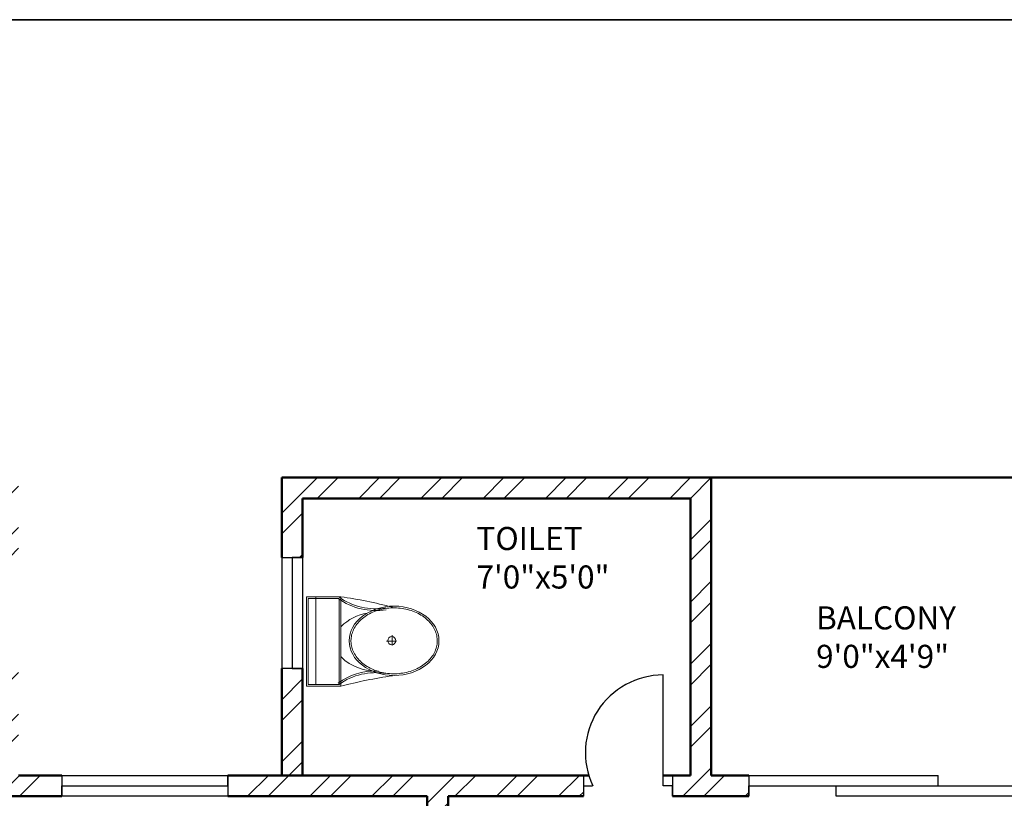
# Model space of a CAD drawing. Units: inches. Extents: x 963 to 2075, y 289 to 2657.
# Tile 97 of 98: x 1672 to 1885, y 2489 to 2657. Entities that reach past the tile are written whole.
import ezdxf

# ---------------------------------------------------------------- set-up
doc = ezdxf.new("R2010")
doc.units = ezdxf.units.IN
for name, color, linetype, lineweight in [('A-ANNO-TTLB', 7, 'Continuous', 35), ('A-AREA-IDEN', 7, 'Continuous', 18), ('A-DOOR', 4, 'Continuous', 25), ('A-FLOR-FIXT', 9, 'Continuous', 18), ('A-GLAZ', 3, 'Continuous', 25), ('A-WALL', 7, 'Continuous', 50), ('A-WALL-PATT', 8, 'Continuous', 13)]:
    doc.layers.add(name, color=color, linetype=linetype, lineweight=lineweight)
doc.styles.get("Standard").update_dxf_attribs({"font": 'arial.ttf'})

# ---------------------------------------------------------------- blocks, each defined once
blk = doc.blocks.new('A$C31115884')
for p, q in [((257.5, 466.4), (257.5, 523.2)), ((283.1, 497.7), (223.4, 497.7)), ((0, 200), (0, 0)), ((520, 200), (0, 200)), ((10, 190), (10, 10)), ((510, 190), (10, 190)), ((510, 10), (510, 190)), ((520, 0), (520, 200)), ((510, 54.5), (0, 54.5)), ((10, 10), (510, 10)), ((0, 0), (520, 0))]:
    blk.add_line(p, q)
blk.add_circle((255.6, 496.4), 23.6)
for centre, radius, start, end in [((2777.7, -204.6), 2807, 165.4549, 171.7133), ((-294.5, 403.3), 364.7, 324.2091, 9.3499), ((-294.5, 403.3), 374.7, 324.2091, 9.3499), ((805.8, 403.3), 364.7, 170.6501, 215.7909), ((3237, 905), 2807, 188.2867, 194.5451), ((139.5, 406.2), 293.5, 315.8436, 2.6563), ((805.8, 403.3), 374.7, 179.2036, 215.7909), ((383.6, 406.2), 293.5, 190.2774, 224.1564)]:
    blk.add_arc(centre, radius, start, end)
blk.add_ellipse((256.2, 509.9), major_axis=(0, -260.7), ratio=0.772727)
blk.add_open_spline([(256.2, 259.2), (263.1, 259.2), (270, 259.7), (287.8, 262.3), (298.7, 265.1), (319.9, 273.1), (330.2, 278.4), (350.1, 291.1), (359.7, 298.7), (377.7, 315.9), (386.2, 325.5), (401.7, 346.6), (408.8, 358.1), (421.3, 382.5), (426.8, 395.5), (435.9, 422.4), (439.5, 436.4), (444.8, 465.1), (446.5, 479.7), (447.9, 509.2), (447.6, 524), (445, 553.3), (442.7, 567.8), (436.3, 596), (432.1, 609.7), (421.9, 636), (416, 648.6), (402.5, 672.1), (395, 683), (378.6, 703), (369.8, 712.1), (351.1, 728), (341.3, 734.8), (320.9, 746.2), (310.4, 750.7), (288.9, 757.3), (278, 759.4), (256, 761), (245, 760.6), (223.1, 757.2), (212.3, 754.3), (191.1, 746.1), (180.8, 740.7), (160.9, 727.8), (151.4, 720.1), (133.5, 702.7), (125.1, 693), (109.6, 671.7), (102.6, 660.2), (90.2, 635.7), (84.9, 622.7), (76, 595.6), (72.4, 581.6), (67.2, 552.9), (65.6, 538.2), (64.4, 508.8), (64.8, 494), (67.5, 464.7), (69.9, 450.2), (76.6, 422), (80.8, 408.3), (91.1, 382.2), (97.2, 369.7), (110.8, 346.3), (118.4, 335.4), (134.8, 315.6), (143.7, 306.7), (162.4, 290.9), (172.3, 284.2), (192.8, 273), (203.3, 268.6), (224.8, 262.2), (235.8, 260.2), (249.9, 259.3), (253, 259.2), (256.2, 259.2)], degree=3, knots=[0, 0, 0, 0, 0.110105, 0.110105, 0.285049, 0.285049, 0.459994, 0.459994, 0.634938, 0.634938, 0.809882, 0.809882, 0.984827, 0.984827, 1.159771, 1.159771, 1.334715, 1.334715, 1.50966, 1.50966, 1.684604, 1.684604, 1.859549, 1.859549, 2.034493, 2.034493, 2.209437, 2.209437, 2.384382, 2.384382, 2.559326, 2.559326, 2.73427, 2.73427, 2.909215, 2.909215, 3.084159, 3.084159, 3.259103, 3.259103, 3.434048, 3.434048, 3.608992, 3.608992, 3.783936, 3.783936, 3.958881, 3.958881, 4.133825, 4.133825, 4.30877, 4.30877, 4.483714, 4.483714, 4.658658, 4.658658, 4.833603, 4.833603, 5.008547, 5.008547, 5.183491, 5.183491, 5.358436, 5.358436, 5.53338, 5.53338, 5.708324, 5.708324, 5.883269, 5.883269, 6.058213, 6.058213, 6.233158, 6.233158, 6.283185, 6.283185, 6.283185, 6.283185])

msp = doc.modelspace()

# ---------------------------------------------------------------- hatches: boundary and pattern name
at = {"layer": 'A-WALL-PATT'}
h = msp.add_hatch(dxfattribs=at)
h.set_pattern_fill('ANSI32', color=256)
h.paths.add_polyline_path([(1296.92, 2558.32), (1203.92, 2558.32), (1203.92, 2493.82), (1191.53, 2493.82), (1191.53, 2489.32), (1211.06, 2489.32), (1211.06, 2492.02), (1211.06, 2493.82), (1208.42, 2493.82), (1208.42, 2553.82), (1292.42, 2553.82), (1292.42, 2538.86), (1296.92, 2538.86)])
h.paths.add_polyline_path([(1442.42, 2558.32), (1349.42, 2558.32), (1349.42, 2538.94), (1353.92, 2538.94), (1353.92, 2553.82), (1437.92, 2553.82), (1437.92, 2493.82), (1434.54, 2493.82), (1434.54, 2489.32), (1448.31, 2489.32), (1448.31, 2491.57), (1448.31, 2493.82), (1442.42, 2493.82)])
h.paths.add_polyline_path([(1415.55, 2491.57), (1415.55, 2493.82), (1340.94, 2493.82), (1340.94, 2489.32), (1371.92, 2489.32), (1371.92, 2378.32), (1367.6, 2378.32), (1367.6, 2373.82), (1371.92, 2373.82), (1371.92, 2355.19), (1376.42, 2355.19), (1376.42, 2489.32), (1415.55, 2489.32)])
h.paths.add_polyline_path([(1304.94, 2491.57), (1304.94, 2493.82), (1296.92, 2493.82), (1296.92, 2514.86), (1292.42, 2514.86), (1292.42, 2493.82), (1232.81, 2493.82), (1232.81, 2489.32), (1256.42, 2489.32), (1256.42, 2327.32), (1253.71, 2327.32), (1253.71, 2322.82), (1328.42, 2322.82), (1328.42, 2331.15), (1323.92, 2331.15), (1323.92, 2327.32), (1260.92, 2327.32), (1260.92, 2373.82), (1323.92, 2373.82), (1323.92, 2357.81), (1328.42, 2357.81), (1328.42, 2373.82), (1346.01, 2373.82), (1346.01, 2376.07), (1346.01, 2378.32), (1260.92, 2378.32), (1260.92, 2489.32), (1304.94, 2489.32)])
h.paths.add_polyline_path([(1226.65, 2327.32), (1124.42, 2327.32), (1124.42, 2347.45), (1119.92, 2347.45), (1119.92, 2322.82), (1163.42, 2322.82), (1163.42, 2305.43), (1165.67, 2305.43), (1167.92, 2305.43), (1167.92, 2322.82), (1226.65, 2322.82), (1226.65, 2325.07)])
h.paths.add_polyline_path([(1095.92, 2489.32), (1124.42, 2489.32), (1131.53, 2489.32), (1131.53, 2491.57), (1131.53, 2493.82), (1119.92, 2493.82), (1091.42, 2493.82), (1091.42, 2417.32), (1095.92, 2417.32), (1119.92, 2417.32), (1119.92, 2407.45), (1124.42, 2407.45), (1124.42, 2421.82), (1095.92, 2421.82)])
h.paths.add_polyline_path([(1512.92, 2558.32), (1508.42, 2558.32), (1508.42, 2493.82), (1503.4, 2493.82), (1503.4, 2489.32), (1508.42, 2489.32), (1508.42, 2327.32), (1376.42, 2327.32), (1376.42, 2330.27), (1371.92, 2330.27), (1371.92, 2298.74), (1376.42, 2298.74), (1376.42, 2322.82), (1508.42, 2322.82), (1508.42, 2165.32), (1504.26, 2165.32), (1504.26, 2160.82), (1508.42, 2160.82), (1508.42, 2108.32), (1512.92, 2108.32), (1512.92, 2160.82), (1516.18, 2160.82), (1516.18, 2163.07), (1516.18, 2165.32), (1512.92, 2165.32), (1512.92, 2322.82), (1644.92, 2322.82), (1644.92, 2298.74), (1649.42, 2298.74), (1649.42, 2322.82), (1649.42, 2330.94), (1647.17, 2330.94), (1644.92, 2330.94), (1644.92, 2327.32), (1512.92, 2327.32), (1512.92, 2489.32), (1516.76, 2489.32), (1516.76, 2491.57), (1516.76, 2493.82), (1512.92, 2493.82)])
h.paths.add_polyline_path([(1671.92, 2558.32), (1578.92, 2558.32), (1578.92, 2493.82), (1573.53, 2493.82), (1573.53, 2489.32), (1586.54, 2489.32), (1586.54, 2491.57), (1586.54, 2493.82), (1583.42, 2493.82), (1583.42, 2553.82), (1667.42, 2553.82), (1667.42, 2541.11), (1671.92, 2541.11)])
h.paths.add_polyline_path([(1681.26, 2493.82), (1671.92, 2493.82), (1671.92, 2517.11), (1667.42, 2517.11), (1667.42, 2493.82), (1610.22, 2493.82), (1610.22, 2489.32), (1644.92, 2489.32), (1644.92, 2357.87), (1649.42, 2357.87), (1649.42, 2373.82), (1652.2, 2373.82), (1652.2, 2375.83), (1652.2, 2378.32), (1649.42, 2378.32), (1649.42, 2489.32), (1681.26, 2489.32), (1681.26, 2491.57)])
h.paths.add_polyline_path([(1821.92, 2558.32), (1728.92, 2558.32), (1728.92, 2541), (1733.42, 2541), (1733.42, 2553.82), (1817.42, 2553.82), (1817.42, 2493.82), (1813.51, 2493.82), (1813.51, 2489.32), (1830.08, 2489.32), (1830.08, 2491.57), (1830.08, 2493.82), (1821.92, 2493.82)])
h.paths.add_polyline_path([(1794.24, 2493.82), (1717.26, 2493.82), (1717.26, 2489.32), (1760.42, 2489.32), (1760.42, 2378.32), (1674.4, 2378.32), (1674.4, 2373.82), (1692.92, 2373.82), (1692.92, 2356.95), (1697.42, 2356.95), (1697.42, 2373.82), (1760.42, 2373.82), (1760.42, 2327.32), (1697.42, 2327.32), (1697.42, 2333.34), (1692.92, 2333.34), (1692.92, 2322.82), (1768.04, 2322.82), (1768.04, 2325.07), (1768.04, 2327.32), (1764.92, 2327.32), (1764.92, 2489.32), (1794.24, 2489.32)])
h.paths.add_polyline_path([(1733.42, 2517), (1728.92, 2517), (1728.92, 2493.82), (1733.42, 2493.82)], flags=17)
h.paths.add_polyline_path([(1929.92, 2493.82), (1890.08, 2493.82), (1890.08, 2489.32), (1896.92, 2489.32), (1925.42, 2489.32), (1925.42, 2421.82), (1896.92, 2421.82), (1896.92, 2408.32), (1901.42, 2408.32), (1901.42, 2417.32), (1925.42, 2417.32), (1929.92, 2417.32)])
h.paths.add_polyline_path([(1901.42, 2348.32), (1896.92, 2348.32), (1896.92, 2327.32), (1800.42, 2327.32), (1800.42, 2322.82), (1853.42, 2322.82), (1853.42, 2309.45), (1857.92, 2309.45), (1857.92, 2322.82), (1901.42, 2322.82)])
h.paths.add_polyline_path([(1857.92, 2249.45), (1853.42, 2249.45), (1853.42, 2214.82), (1686.31, 2214.82), (1686.31, 2210.32), (1853.42, 2210.32), (1853.42, 2202.13), (1857.92, 2202.13), (1857.92, 2210.32)])
h.paths.add_polyline_path([(1857.92, 2142.13), (1853.42, 2142.13), (1853.42, 2115.42), (1841.42, 2115.42), (1841.42, 2088.53), (1841.42, 2046.95), (1845.92, 2046.95), (1845.92, 2110.92), (1905.92, 2110.92), (1905.92, 2092.52), (1910.42, 2092.52), (1910.42, 2115.42), (1857.92, 2115.42)])
h.paths.add_polyline_path([(1532.44, 1482.34), (1573.46, 1482.34), (1573.46, 1501), (1532.44, 1501)], flags=9)
h.paths.add_polyline_path([(1438.66, 1486.3), (1479.68, 1486.3), (1479.68, 1504.96), (1438.66, 1504.96)], flags=9)
h.paths.add_polyline_path([(1411.22, 1365.31), (1659.14, 1365.31), (1659.14, 1402.4), (1411.22, 1402.4)], flags=9)
h.paths.add_polyline_path([(1185.67, 2296.3), (1248.16, 2296.3), (1248.16, 2314.95), (1185.67, 2314.95)], flags=9)
h.paths.add_polyline_path([(1177.31, 2187.35), (1216.15, 2187.35), (1216.15, 2206.01), (1177.31, 2206.01)], flags=9)
h.paths.add_polyline_path([(1295.1, 1602.08), (1328.26, 1602.08), (1328.26, 1620.74), (1295.1, 1620.74)], flags=9)
h.paths.add_polyline_path([(1525.13, 2005.99), (1558.39, 2005.99), (1558.39, 2024.65), (1525.13, 2024.65)], flags=9)
h.paths.add_polyline_path([(1459.61, 1977.13), (1472.19, 1977.13), (1472.19, 1987.43), (1459.61, 1987.43)], flags=9)
h.paths.add_polyline_path([(1467.81, 2053.68), (1480.02, 2053.68), (1480.02, 2063.98), (1467.81, 2063.98)], flags=9)
h.paths.add_polyline_path([(1555.18, 2119.02), (1584.56, 2119.02), (1584.56, 2137.68), (1555.18, 2137.68)], flags=25)
h.paths.add_polyline_path([(1405.39, 2115.29), (1444.48, 2115.29), (1444.48, 2133.95), (1405.39, 2133.95)], flags=25)
h.paths.add_polyline_path([(1698.48, 2004.26), (1727.69, 2004.26), (1727.69, 2022.92), (1698.48, 2022.92)], flags=9)
h.paths.add_polyline_path([(1612.16, 1972.86), (1629.02, 1972.86), (1629.02, 1983.16), (1612.16, 1983.16)], flags=9)
h.paths.add_polyline_path([(1608.29, 2060.04), (1625.15, 2060.04), (1625.15, 2070.34), (1608.29, 2070.34)], flags=9)
h.paths.add_polyline_path([(1527.95, 1684.4), (1566.79, 1684.4), (1566.79, 1703.06), (1527.95, 1703.06)], flags=9)
h.paths.add_polyline_path([(1422.79, 1683.59), (1461.63, 1683.59), (1461.63, 1702.25), (1422.79, 1702.25)], flags=9)
h.paths.add_polyline_path([(1531.26, 1732.46), (1574.01, 1732.46), (1574.01, 1751.12), (1531.26, 1751.12)], flags=9)
h.paths.add_polyline_path([(1402.87, 1732.85), (1439.8, 1732.85), (1439.8, 1751.5), (1402.87, 1751.5)], flags=9)
h.paths.add_polyline_path([(1243.12, 1923.13), (1281.96, 1923.13), (1281.96, 1941.79), (1243.12, 1941.79)], flags=9)
h.paths.add_polyline_path([(1181.75, 1792.27), (1244.24, 1792.27), (1244.24, 1810.93), (1181.75, 1810.93)], flags=9)
h.paths.add_polyline_path([(1265.82, 1670.3), (1316.07, 1670.3), (1316.07, 1688.96), (1265.82, 1688.96)], flags=9)
h.paths.add_polyline_path([(1140.26, 1676.05), (1179.1, 1676.05), (1179.1, 1694.71), (1140.26, 1694.71)], flags=9)
h.paths.add_polyline_path([(1107.49, 1490.89), (1143.37, 1490.89), (1143.37, 1509.55), (1107.49, 1509.55)], flags=9)
h.paths.add_polyline_path([(1217.58, 1483.9), (1246.74, 1483.9), (1246.74, 1502.56), (1217.58, 1502.56)], flags=9)
h.paths.add_polyline_path([(1389.21, 1486.92), (1418.37, 1486.92), (1418.37, 1505.58), (1389.21, 1505.58)], flags=9)
h.paths.add_polyline_path([(1672.21, 1602.08), (1705.37, 1602.08), (1705.37, 1620.74), (1672.21, 1620.74)], flags=9)
h.paths.add_polyline_path([(1752.08, 1522.64), (1781.24, 1522.64), (1781.24, 1541.3), (1752.08, 1541.3)], flags=9)
h.paths.add_polyline_path([(1848.27, 1491.26), (1884.16, 1491.26), (1884.16, 1509.92), (1848.27, 1509.92)], flags=9)
h.paths.add_polyline_path([(1822.47, 1685.62), (1861.31, 1685.62), (1861.31, 1704.28), (1822.47, 1704.28)], flags=9)
h.paths.add_polyline_path([(1713.19, 1672.23), (1763.44, 1672.23), (1763.44, 1690.89), (1713.19, 1690.89)], flags=9)
h.paths.add_polyline_path([(1736.62, 1790.58), (1799.11, 1790.58), (1799.11, 1809.24), (1736.62, 1809.24)], flags=9)
h.paths.add_polyline_path([(1691.49, 1916.36), (1730.33, 1916.36), (1730.33, 1935.01), (1691.49, 1935.01)], flags=9)
h.paths.add_polyline_path([(1764.87, 1973.92), (1794.31, 1973.92), (1794.31, 1992.58), (1764.87, 1992.58)], flags=9)
h.paths.add_polyline_path([(1767.85, 2034.02), (1797.29, 2034.02), (1797.29, 2052.67), (1767.85, 2052.67)], flags=9)
h.paths.add_polyline_path([(1851.59, 2060.33), (1880.75, 2060.33), (1880.75, 2078.99), (1851.59, 2078.99)], flags=25)
h.paths.add_polyline_path([(1688.49, 2086.87), (1727.33, 2086.87), (1727.33, 2105.53), (1688.49, 2105.53)], flags=9)
h.paths.add_polyline_path([(1537.74, 2293.58), (1580.49, 2293.58), (1580.49, 2312.24), (1537.74, 2312.24)], flags=25)
h.paths.add_polyline_path([(1425.59, 2296.11), (1468.34, 2296.11), (1468.34, 2314.77), (1425.59, 2314.77)], flags=25)
h.paths.add_polyline_path([(1278.52, 2004.18), (1307.72, 2004.18), (1307.72, 2022.84), (1278.52, 2022.84)], flags=9)
h.paths.add_polyline_path([(1193.28, 1973.63), (1222.72, 1973.63), (1222.72, 1992.29), (1193.28, 1992.29)], flags=9)
h.paths.add_polyline_path([(1192.41, 2040.58), (1221.84, 2040.58), (1221.84, 2059.23), (1192.41, 2059.23)], flags=9)
h.paths.add_polyline_path([(1130.6, 1951.39), (1159.76, 1951.39), (1159.76, 1970.05), (1130.6, 1970.05)], flags=9)
h.paths.add_polyline_path([(1132.83, 2052.49), (1161.98, 2052.49), (1161.98, 2071.15), (1132.83, 2071.15)], flags=9)
h.paths.add_polyline_path([(1265.13, 2334.62), (1315.38, 2334.62), (1315.38, 2353.28), (1265.13, 2353.28)], flags=25)
h.paths.add_polyline_path([(1136.74, 2330.79), (1175.58, 2330.79), (1175.58, 2349.44), (1136.74, 2349.44)], flags=9)
h.paths.add_polyline_path([(1287.42, 2417.2), (1320.58, 2417.2), (1320.58, 2435.86), (1287.42, 2435.86)], flags=25)
h.paths.add_polyline_path([(1430.99, 2329.16), (1469.83, 2329.16), (1469.83, 2347.82), (1430.99, 2347.82)], flags=25)
h.paths.add_polyline_path([(1525.42, 2329.21), (1564.26, 2329.21), (1564.26, 2347.87), (1525.42, 2347.87)], flags=25)
h.paths.add_polyline_path([(1684.52, 2382.8), (1717.68, 2382.8), (1717.68, 2401.46), (1684.52, 2401.46)], flags=25)
h.paths.add_polyline_path([(1704.81, 2340.29), (1755.05, 2340.29), (1755.05, 2358.95), (1704.81, 2358.95)], flags=25)
h.paths.add_polyline_path([(1694.11, 2287.76), (1756.6, 2287.76), (1756.6, 2306.41), (1694.11, 2306.41)], flags=9)
h.paths.add_polyline_path([(1815.78, 2329.86), (1854.62, 2329.86), (1854.62, 2348.52), (1815.78, 2348.52)], flags=9)
h.paths.add_polyline_path([(1842.87, 2514.26), (1878.76, 2514.26), (1878.76, 2532.91), (1842.87, 2532.91)], flags=9)
h.paths.add_polyline_path([(1769.51, 2531.45), (1798.67, 2531.45), (1798.67, 2550.1), (1769.51, 2550.1)], flags=25)
h.paths.add_polyline_path([(1594.77, 2518.47), (1623.93, 2518.47), (1623.93, 2537.13), (1594.77, 2537.13)], flags=25)
h.paths.add_polyline_path([(1520.72, 2516.18), (1556.61, 2516.18), (1556.61, 2534.84), (1520.72, 2534.84)], flags=25)
h.paths.add_polyline_path([(1464.46, 2516.69), (1500.34, 2516.69), (1500.34, 2535.35), (1464.46, 2535.35)], flags=25)
h.paths.add_polyline_path([(1365.7, 2528.97), (1394.85, 2528.97), (1394.85, 2547.63), (1365.7, 2547.63)], flags=25)
h.paths.add_polyline_path([(1222.84, 2516.23), (1252, 2516.23), (1252, 2534.89), (1222.84, 2534.89)], flags=25)
h.paths.add_polyline_path([(1104.55, 2509.6), (1140.43, 2509.6), (1140.43, 2528.26), (1104.55, 2528.26)], flags=9)
h = msp.add_hatch(dxfattribs=at)
h.set_pattern_fill('ANSI32', color=256)
h.paths.add_polyline_path([(1335.97, 2212.57), (1335.97, 2214.82), (1167.92, 2214.82), (1167.92, 2245.43), (1163.42, 2245.43), (1163.42, 2210.32), (1163.42, 2194.81), (1167.92, 2194.81), (1167.92, 2210.32), (1335.97, 2210.32)])
h.paths.add_polyline_path([(1532.44, 1482.34), (1573.46, 1482.34), (1573.46, 1501), (1532.44, 1501)], flags=9)
h.paths.add_polyline_path([(1438.66, 1486.3), (1479.68, 1486.3), (1479.68, 1504.96), (1438.66, 1504.96)], flags=9)
h.paths.add_polyline_path([(1411.22, 1365.31), (1659.14, 1365.31), (1659.14, 1402.4), (1411.22, 1402.4)], flags=9)
h.paths.add_polyline_path([(1185.67, 2296.3), (1248.16, 2296.3), (1248.16, 2314.95), (1185.67, 2314.95)], flags=9)
h.paths.add_polyline_path([(1177.31, 2187.35), (1216.15, 2187.35), (1216.15, 2206.01), (1177.31, 2206.01)], flags=9)
h.paths.add_polyline_path([(1295.1, 1602.08), (1328.26, 1602.08), (1328.26, 1620.74), (1295.1, 1620.74)], flags=9)
h.paths.add_polyline_path([(1525.13, 2005.99), (1558.39, 2005.99), (1558.39, 2024.65), (1525.13, 2024.65)], flags=9)
h.paths.add_polyline_path([(1459.61, 1977.13), (1472.19, 1977.13), (1472.19, 1987.43), (1459.61, 1987.43)], flags=9)
h.paths.add_polyline_path([(1467.81, 2053.68), (1480.02, 2053.68), (1480.02, 2063.98), (1467.81, 2063.98)], flags=9)
h.paths.add_polyline_path([(1555.18, 2119.02), (1584.56, 2119.02), (1584.56, 2137.68), (1555.18, 2137.68)], flags=9)
h.paths.add_polyline_path([(1405.39, 2115.29), (1444.48, 2115.29), (1444.48, 2133.95), (1405.39, 2133.95)], flags=9)
h.paths.add_polyline_path([(1698.48, 2004.26), (1727.69, 2004.26), (1727.69, 2022.92), (1698.48, 2022.92)], flags=9)
h.paths.add_polyline_path([(1612.16, 1972.86), (1629.02, 1972.86), (1629.02, 1983.16), (1612.16, 1983.16)], flags=9)
h.paths.add_polyline_path([(1608.29, 2060.04), (1625.15, 2060.04), (1625.15, 2070.34), (1608.29, 2070.34)], flags=9)
h.paths.add_polyline_path([(1527.95, 1684.4), (1566.79, 1684.4), (1566.79, 1703.06), (1527.95, 1703.06)], flags=9)
h.paths.add_polyline_path([(1422.79, 1683.59), (1461.63, 1683.59), (1461.63, 1702.25), (1422.79, 1702.25)], flags=9)
h.paths.add_polyline_path([(1531.26, 1732.46), (1574.01, 1732.46), (1574.01, 1751.12), (1531.26, 1751.12)], flags=9)
h.paths.add_polyline_path([(1402.87, 1732.85), (1439.8, 1732.85), (1439.8, 1751.5), (1402.87, 1751.5)], flags=9)
h.paths.add_polyline_path([(1243.12, 1923.13), (1281.96, 1923.13), (1281.96, 1941.79), (1243.12, 1941.79)], flags=9)
h.paths.add_polyline_path([(1181.75, 1792.27), (1244.24, 1792.27), (1244.24, 1810.93), (1181.75, 1810.93)], flags=9)
h.paths.add_polyline_path([(1265.82, 1670.3), (1316.07, 1670.3), (1316.07, 1688.96), (1265.82, 1688.96)], flags=9)
h.paths.add_polyline_path([(1140.26, 1676.05), (1179.1, 1676.05), (1179.1, 1694.71), (1140.26, 1694.71)], flags=9)
h.paths.add_polyline_path([(1107.49, 1490.89), (1143.37, 1490.89), (1143.37, 1509.55), (1107.49, 1509.55)], flags=9)
h.paths.add_polyline_path([(1217.58, 1483.9), (1246.74, 1483.9), (1246.74, 1502.56), (1217.58, 1502.56)], flags=9)
h.paths.add_polyline_path([(1389.21, 1486.92), (1418.37, 1486.92), (1418.37, 1505.58), (1389.21, 1505.58)], flags=9)
h.paths.add_polyline_path([(1672.21, 1602.08), (1705.37, 1602.08), (1705.37, 1620.74), (1672.21, 1620.74)], flags=9)
h.paths.add_polyline_path([(1752.08, 1522.64), (1781.24, 1522.64), (1781.24, 1541.3), (1752.08, 1541.3)], flags=9)
h.paths.add_polyline_path([(1848.27, 1491.26), (1884.16, 1491.26), (1884.16, 1509.92), (1848.27, 1509.92)], flags=9)
h.paths.add_polyline_path([(1822.47, 1685.62), (1861.31, 1685.62), (1861.31, 1704.28), (1822.47, 1704.28)], flags=9)
h.paths.add_polyline_path([(1713.19, 1672.23), (1763.44, 1672.23), (1763.44, 1690.89), (1713.19, 1690.89)], flags=9)
h.paths.add_polyline_path([(1736.62, 1790.58), (1799.11, 1790.58), (1799.11, 1809.24), (1736.62, 1809.24)], flags=9)
h.paths.add_polyline_path([(1691.49, 1916.36), (1730.33, 1916.36), (1730.33, 1935.01), (1691.49, 1935.01)], flags=9)
h.paths.add_polyline_path([(1764.87, 1973.92), (1794.31, 1973.92), (1794.31, 1992.58), (1764.87, 1992.58)], flags=9)
h.paths.add_polyline_path([(1767.85, 2034.02), (1797.29, 2034.02), (1797.29, 2052.67), (1767.85, 2052.67)], flags=9)
h.paths.add_polyline_path([(1851.59, 2060.33), (1880.75, 2060.33), (1880.75, 2078.99), (1851.59, 2078.99)], flags=9)
h.paths.add_polyline_path([(1688.49, 2086.87), (1727.33, 2086.87), (1727.33, 2105.53), (1688.49, 2105.53)], flags=9)
h.paths.add_polyline_path([(1537.74, 2293.58), (1580.49, 2293.58), (1580.49, 2312.24), (1537.74, 2312.24)], flags=9)
h.paths.add_polyline_path([(1425.59, 2296.11), (1468.34, 2296.11), (1468.34, 2314.77), (1425.59, 2314.77)], flags=9)
h.paths.add_polyline_path([(1278.52, 2004.18), (1307.72, 2004.18), (1307.72, 2022.84), (1278.52, 2022.84)], flags=9)
h.paths.add_polyline_path([(1193.28, 1973.63), (1222.72, 1973.63), (1222.72, 1992.29), (1193.28, 1992.29)], flags=9)
h.paths.add_polyline_path([(1192.41, 2040.58), (1221.84, 2040.58), (1221.84, 2059.23), (1192.41, 2059.23)], flags=9)
h.paths.add_polyline_path([(1130.6, 1951.39), (1159.76, 1951.39), (1159.76, 1970.05), (1130.6, 1970.05)], flags=9)
h.paths.add_polyline_path([(1132.83, 2052.49), (1161.98, 2052.49), (1161.98, 2071.15), (1132.83, 2071.15)], flags=9)
h.paths.add_polyline_path([(1265.13, 2334.62), (1315.38, 2334.62), (1315.38, 2353.28), (1265.13, 2353.28)], flags=9)
h.paths.add_polyline_path([(1136.74, 2330.79), (1175.58, 2330.79), (1175.58, 2349.44), (1136.74, 2349.44)], flags=9)
h.paths.add_polyline_path([(1287.42, 2417.2), (1320.58, 2417.2), (1320.58, 2435.86), (1287.42, 2435.86)], flags=9)
h.paths.add_polyline_path([(1430.99, 2329.16), (1469.83, 2329.16), (1469.83, 2347.82), (1430.99, 2347.82)], flags=9)
h.paths.add_polyline_path([(1525.42, 2329.21), (1564.26, 2329.21), (1564.26, 2347.87), (1525.42, 2347.87)], flags=9)
h.paths.add_polyline_path([(1684.52, 2382.8), (1717.68, 2382.8), (1717.68, 2401.46), (1684.52, 2401.46)], flags=9)
h.paths.add_polyline_path([(1704.81, 2340.29), (1755.05, 2340.29), (1755.05, 2358.95), (1704.81, 2358.95)], flags=9)
h.paths.add_polyline_path([(1694.11, 2287.76), (1756.6, 2287.76), (1756.6, 2306.41), (1694.11, 2306.41)], flags=9)
h.paths.add_polyline_path([(1815.78, 2329.86), (1854.62, 2329.86), (1854.62, 2348.52), (1815.78, 2348.52)], flags=9)
h.paths.add_polyline_path([(1842.87, 2514.26), (1878.76, 2514.26), (1878.76, 2532.91), (1842.87, 2532.91)], flags=9)
h.paths.add_polyline_path([(1769.51, 2531.45), (1798.67, 2531.45), (1798.67, 2550.1), (1769.51, 2550.1)], flags=9)
h.paths.add_polyline_path([(1594.77, 2518.47), (1623.93, 2518.47), (1623.93, 2537.13), (1594.77, 2537.13)], flags=9)
h.paths.add_polyline_path([(1520.72, 2516.18), (1556.61, 2516.18), (1556.61, 2534.84), (1520.72, 2534.84)], flags=9)
h.paths.add_polyline_path([(1464.46, 2516.69), (1500.34, 2516.69), (1500.34, 2535.35), (1464.46, 2535.35)], flags=9)
h.paths.add_polyline_path([(1365.7, 2528.97), (1394.85, 2528.97), (1394.85, 2547.63), (1365.7, 2547.63)], flags=9)
h.paths.add_polyline_path([(1222.84, 2516.23), (1252, 2516.23), (1252, 2534.89), (1222.84, 2534.89)], flags=9)
h.paths.add_polyline_path([(1104.55, 2509.6), (1140.43, 2509.6), (1140.43, 2528.26), (1104.55, 2528.26)], flags=9)

# ---------------------------------------------------------------- linework, layer by layer
at = {"layer": 'A-ANNO-TTLB'}
msp.add_lwpolyline([(962.81, 2657.49), (2074.6, 2657.49), (2074.6, 1303.08), (962.81, 1303.08)], close=True, dxfattribs=at)
at = {"layer": 'A-DOOR'}
for p, q in [((1811.51, 2491.57), (1811.51, 2515.57)), ((1794.24, 2493.82), (1794.24, 2489.32)), ((1813.51, 2493.82), (1813.51, 2489.32)), ((1794.24, 2491.57), (1796.24, 2491.57)), ((1813.51, 2491.57), (1811.51, 2491.57)), ((1813.51, 2489.32), (1813.51, 2491.57))]:
    msp.add_line(p, q, dxfattribs=at)
msp.add_arc((1811.51, 2498.71), 16.85, 90, 205.0881, dxfattribs=at)
at = {"layer": 'A-GLAZ'}
for p, q in [((1728.92, 2541), (1733.42, 2541)), ((1728.92, 2541), (1728.92, 2517)), ((1733.42, 2541), (1731.17, 2541)), ((1731.17, 2541), (1731.17, 2517)), ((1733.42, 2541), (1733.42, 2517)), ((1733.42, 2517), (1728.92, 2517)), ((1731.17, 2517), (1733.42, 2517)), ((1681.26, 2493.82), (1681.26, 2489.32)), ((1681.26, 2493.82), (1717.26, 2493.82)), ((1717.26, 2491.57), (1717.26, 2493.82)), ((1717.26, 2493.82), (1717.26, 2489.32)), ((1830.08, 2493.82), (1830.08, 2489.32)), ((1830.08, 2493.82), (1871.09, 2493.82)), ((1871.09, 2491.57), (1871.09, 2493.82)), ((1681.26, 2489.32), (1681.26, 2491.57)), ((1681.26, 2491.57), (1717.26, 2491.57)), ((1830.08, 2489.32), (1830.08, 2491.57)), ((1830.08, 2491.57), (1890.08, 2491.57)), ((1848.98, 2489.32), (1848.98, 2491.57)), ((1717.26, 2489.32), (1681.26, 2489.32)), ((1890.08, 2489.32), (1848.98, 2489.32))]:
    msp.add_line(p, q, dxfattribs=at)
at = {"layer": 'A-WALL'}
for p, q in [((1728.92, 2558.32), (1929.92, 2558.32)), ((1728.92, 2541), (1728.92, 2558.32)), ((1821.92, 2558.32), (1821.92, 2493.82)), ((1817.42, 2553.82), (1733.42, 2553.82)), ((1733.42, 2541), (1733.42, 2553.82)), ((1817.42, 2493.82), (1817.42, 2553.82)), ((1728.92, 2493.82), (1728.92, 2517)), ((1733.42, 2493.82), (1733.42, 2517)), ((1671.92, 2493.82), (1681.26, 2493.82)), ((1717.26, 2493.82), (1795.38, 2493.82)), ((1811.51, 2493.82), (1817.42, 2493.82)), ((1821.92, 2493.82), (1830.08, 2493.82)), ((1821.92, 2493.82), (1830.08, 2493.82)), ((1649.42, 2489.32), (1681.26, 2489.32)), ((1717.26, 2489.32), (1760.42, 2489.32)), ((1760.42, 2489.32), (1760.42, 2378.32)), ((1764.92, 2489.32), (1764.92, 2327.32)), ((1764.92, 2489.32), (1794.24, 2489.32)), ((1813.51, 2489.32), (1830.08, 2489.32))]:
    msp.add_line(p, q, dxfattribs=at)

# ---------------------------------------------------------------- block references
at = {"layer": 'A-FLOR-FIXT', "xscale": 0.0372717239612423, "yscale": 0.0372717239612423, "zscale": 0.0372717239612423, "rotation": 270}
msp.add_blockref('A$C31115884', (1734.24, 2532.51), dxfattribs=at)

# ---------------------------------------------------------------- texts
at = {"layer": 'A-AREA-IDEN', "char_height": 5, "attachment_point": 1}
for s, width, insert in [('TOILET\\P7\'0"x5\'0"', 104.7373, (1771.09, 2547.62)), ('BALCONY\\P9\'0"x4\'9"', 186.1372, (1844.63, 2530.43))]:
    msp.add_mtext_dynamic_manual_height_columns(s, width=width, gutter_width=12.5, heights=[0], dxfattribs=dict(at, insert=insert))

doc.saveas('drawing.dxf')
